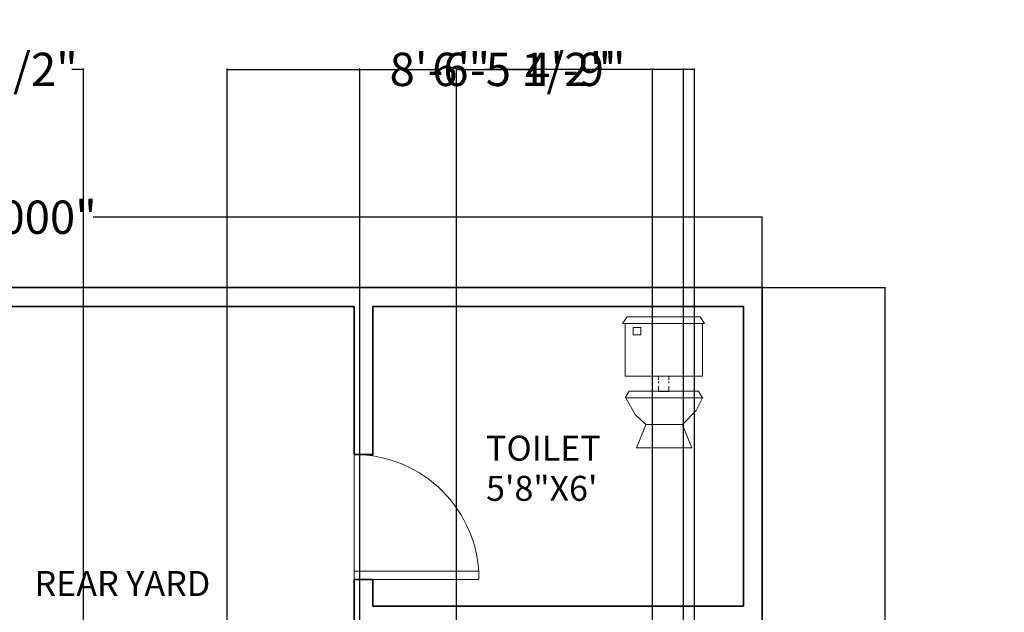
# Model space of a CAD drawing. Units: inches. Extents: x -438 to 102, y -60 to 1091.
# Tile 20 of 20: x -149 to 87, y 949 to 1091. Entities that reach past the tile are written whole.
import ezdxf

# ---------------------------------------------------------------- set-up
doc = ezdxf.new("R2010")
doc.units = ezdxf.units.IN
doc.header["$MEASUREMENT"] = 0
for name, color, linetype, lineweight, true_color in [('A-ANNO-DIMS', 217, 'Continuous', 18, 0x93278f), ('A-DOOR', 30, 'Continuous', 18, 0xf26722), ('A-WALL', 2, 'Continuous', 35, 0xf1eb1f), ('C-PROP', 2, 'Continuous', 35, 0xf1eb1f)]:
    doc.layers.add(name, color=color, linetype=linetype, lineweight=lineweight, true_color=true_color)
doc.layers.add('A-AREA-IDEN', color=4, linetype='Continuous', lineweight=18)
doc.layers.add('A-FLOR-FIXT', color=9, linetype='Continuous', lineweight=15)
doc.styles.get("Standard").update_dxf_attribs({"font": 'arial.ttf'})
doc.dimstyles.get("Standard").update_dxf_attribs({"dimtxt": 8, "dimasz": 0.18, "dimexe": 0.18, "dimexo": 0.0625, "dimgap": 0.09, "dimtad": 0, "dimtih": 1, "dimtoh": 1, "dimdec": 4, "dimzin": 0, "dimdsep": 46, "dimlunit": 3, "dimtxsty": 'Standard', "dimcen": 0.09, "dimadec": 0, "dimazin": 0, "dimtfac": 1, "dimtdec": 4, "dimtofl": 0, "dimtmove": 0, "dimatfit": 3, "dimfxl": 1, "dimtolj": 1, "dimtzin": 0, "dimarcsym": 0})

# ---------------------------------------------------------------- blocks, each defined once
blk = doc.blocks.new('*D4')
at = {"layer": 'A-ANNO-DIMS', "color": 0, "lineweight": -2, "transparency": 16777216}
for p, q in [((-354.15, 1027.06), (-354.15, 1044.09)), ((-353.97, 1043.91), (-193.57, 1043.91)), ((28.67, 1043.91), (-131.73, 1043.91)), ((28.85, 1027.06), (28.85, 1044.09))]:
    blk.add_line(p, q, dxfattribs=at)
at = {"layer": 'A-ANNO-DIMS', "color": 0, "transparency": 16777216}
for points in [[(-353.97, 1043.94), (-353.97, 1043.88), (-354.15, 1043.91)], [(28.67, 1043.94), (28.67, 1043.88), (28.85, 1043.91)]]:
    blk.add_solid(points, dxfattribs=at)
at = {"layer": 'Defpoints', "color": 0, "transparency": 16777216}
for p in [(28.85, 1043.91), (-354.15, 1027), (28.85, 1027)]:
    blk.add_point(p, dxfattribs=at)
at = {"layer": 'A-ANNO-DIMS', "color": 0, "transparency": 16777216, "insert": (-162.65, 1043.91), "char_height": 8, "attachment_point": 5}
blk.add_mtext('\\A1;31\'-11.0000"', dxfattribs=at)
blk = doc.blocks.new('*D5')
at = {"layer": 'A-ANNO-DIMS', "color": 0, "lineweight": -2, "transparency": 16777216}
for p, q in [((28.92, 1027), (58.42, 1027)), ((58.24, 1026.82), (58.24, 519.68)), ((58.24, 4.18), (58.24, 511.32)), ((28.92, 4), (58.42, 4))]:
    blk.add_line(p, q, dxfattribs=at)
at = {"layer": 'A-ANNO-DIMS', "color": 0, "transparency": 16777216}
for points in [[(58.21, 1026.82), (58.27, 1026.82), (58.24, 1027)], [(58.21, 4.18), (58.27, 4.18), (58.24, 4)]]:
    blk.add_solid(points, dxfattribs=at)
at = {"layer": 'Defpoints', "color": 0, "transparency": 16777216}
for p in [(28.85, 1027), (28.85, 4), (58.24, 4)]:
    blk.add_point(p, dxfattribs=at)
at = {"layer": 'A-ANNO-DIMS', "color": 0, "transparency": 16777216, "insert": (58.24, 515.5), "char_height": 8, "attachment_point": 5}
blk.add_mtext('\\A1;85\'-3.0000"', dxfattribs=at)
blk = doc.blocks.new('WC-CLOSE-COUPLED')
for p, q in [((-9.84, -1.66, -13.5), (-8.74, 0, -13.5)), ((-8.74, 0, -13.5), (8.78, 0, -13.5)), ((9.84, -1.66, -13.5), (8.78, 0, -13.5)), ((-9.84, -1.66, -13.5), (9.84, -1.66, -13.5)), ((-9.27, -1.66, -13.5), (-9.27, -14.26, -13.5)), ((9.31, -14.26, -13.5), (9.31, -1.66, -13.5)), ((-7.35, -2.62, -13.5), (-7.35, -4.39, -13.5)), ((-5.45, -2.62, -13.5), (-7.35, -2.62, -13.5)), ((-7.35, -4.39, -13.5), (-5.45, -4.39, -13.5)), ((-5.45, -4.39, -13.5), (-5.45, -2.62, -13.5)), ((-9.27, -14.26, -13.5), (9.31, -14.26, -13.5)), ((-1.22, -15.15, -13.5), (-1.22, -14.23, -13.5)), ((-1.22, -15.97, -13.5), (-1.22, -15.56, -13.5)), ((0.02, -14.26, -13.5), (1.26, -14.26, -13.5)), ((1.26, -14.26, -13.5), (1.26, -15.15, -13.5)), ((1.26, -15.56, -13.5), (1.26, -15.97, -13.5)), ((-9.27, -19.49, -13.5), (-8.25, -17.89, -13.5)), ((-8.25, -17.89, -13.5), (8.4, -17.89, -13.5)), ((-1.22, -17.96, -13.5), (-1.22, -16.65, -13.5)), ((1.26, -17.96, -13.5), (-1.22, -17.96, -13.5)), ((1.26, -16.65, -13.5), (1.26, -17.96, -13.5)), ((9.31, -19.49, -13.5), (8.4, -17.89, -13.5)), ((-9.27, -19.49, -13.5), (9.31, -19.49, -13.5)), ((9.52, -19.49, -13.5), (-9.07, -19.49, -13.5)), ((-9.07, -19.49, -13.5), (-6.87, -23.48, -13.5)), ((7.85, -22.5, -13.5), (9.31, -19.49, -13.5)), ((-6.87, -23.48, -13.5), (-4.26, -25.89, -13.5)), ((4.51, -25.89, -13.5), (7.85, -22.5, -13.5)), ((-6.51, -31.49, -13.5), (-4.3, -25.95, -13.5)), ((-4.26, -25.89, -13.5), (4.51, -25.89, -13.5)), ((4.51, -25.89, -13.5), (-4.26, -25.89, -13.5)), ((6.76, -31.49, -13.5), (4.55, -25.95, -13.5)), ((-6.51, -31.49, -13.5), (6.76, -31.49, -13.5)), ((0.12, -31.49, -13.5), (-6.51, -31.49, -13.5))]:
    blk.add_line(p, q)
blk = doc.blocks.new('DOOR-SWING-30')
for p, q in [((0, 0), (-30, 0)), ((0, -30), (0, 0)), ((0, -2), (-30, -2))]:
    blk.add_line(p, q)
blk.add_arc((0, 0), 30, 180, 270)
blk = doc.blocks.new('*D37')
at = {"layer": 'A-ANNO-DIMS', "color": 0, "lineweight": -2, "transparency": 16777216}
for p, q in [((-179.8, 234.94), (-179.8, 1079.58)), ((-179.62, 1079.4), (-176.98, 1079.4)), ((-134.26, 1079.4), (-136.9, 1079.4)), ((-134.08, 234.94), (-134.08, 1079.58))]:
    blk.add_line(p, q, dxfattribs=at)
at = {"layer": 'A-ANNO-DIMS', "color": 0, "transparency": 16777216}
for points in [[(-179.62, 1079.43), (-179.62, 1079.37), (-179.8, 1079.4)], [(-134.26, 1079.43), (-134.26, 1079.37), (-134.08, 1079.4)]]:
    blk.add_solid(points, dxfattribs=at)
at = {"layer": 'Defpoints', "color": 0, "transparency": 16777216}
for p in [(-134.08, 1079.4), (-179.8, 234.88), (-134.08, 234.88)]:
    blk.add_point(p, dxfattribs=at)
at = {"layer": 'A-ANNO-DIMS', "color": 0, "transparency": 16777216, "insert": (-156.94, 1079.4), "char_height": 8, "attachment_point": 5}
blk.add_mtext('\\A1;3\'-9 1/2"', dxfattribs=at)
blk = doc.blocks.new('*D45')
at = {"layer": 'A-ANNO-DIMS', "color": 0, "lineweight": -2, "transparency": 16777216}
for p, q in [((-99.58, 615.92), (-99.58, 1079.58)), ((-99.4, 1079.4), (-59.27, 1079.4)), ((2.32, 1079.4), (-37.82, 1079.4)), ((2.5, 615.92), (2.5, 1079.58))]:
    blk.add_line(p, q, dxfattribs=at)
at = {"layer": 'A-ANNO-DIMS', "color": 0, "transparency": 16777216}
for points in [[(-99.4, 1079.43), (-99.4, 1079.37), (-99.58, 1079.4)], [(2.32, 1079.43), (2.32, 1079.37), (2.5, 1079.4)]]:
    blk.add_solid(points, dxfattribs=at)
at = {"layer": 'Defpoints', "color": 0, "transparency": 16777216}
for p in [(2.5, 1079.4), (-99.58, 615.86), (2.5, 615.86)]:
    blk.add_point(p, dxfattribs=at)
at = {"layer": 'A-ANNO-DIMS', "color": 0, "transparency": 16777216, "insert": (-48.54, 1079.4), "char_height": 8, "attachment_point": 5}
blk.add_mtext('\\A1;8\'-6"', dxfattribs=at)
blk = doc.blocks.new('*D47')
at = {"layer": 'A-ANNO-DIMS', "color": 0, "lineweight": -2, "transparency": 16777216}
for p, q in [((-67.74, 529.33), (-67.74, 1079.58)), ((-67.56, 1079.4), (-48.98, 1079.4)), ((9.73, 1079.4), (-8.85, 1079.4)), ((9.91, 529.33), (9.91, 1079.58))]:
    blk.add_line(p, q, dxfattribs=at)
at = {"layer": 'A-ANNO-DIMS', "color": 0, "transparency": 16777216}
for points in [[(-67.56, 1079.43), (-67.56, 1079.37), (-67.74, 1079.4)], [(9.73, 1079.43), (9.73, 1079.37), (9.91, 1079.4)]]:
    blk.add_solid(points, dxfattribs=at)
at = {"layer": 'Defpoints', "color": 0, "transparency": 16777216}
for p in [(9.91, 1079.4), (-67.74, 529.27), (9.91, 529.27)]:
    blk.add_point(p, dxfattribs=at)
at = {"layer": 'A-ANNO-DIMS', "color": 0, "transparency": 16777216, "insert": (-28.91, 1079.4), "char_height": 8, "attachment_point": 5}
blk.add_mtext('\\A1;6\'-5 1/2"', dxfattribs=at)
blk = doc.blocks.new('*D49')
at = {"layer": 'A-ANNO-DIMS', "color": 0, "lineweight": -2, "transparency": 16777216}
for p, q in [((-44.57, 339.86), (-44.57, 1079.58)), ((-44.39, 1079.4), (-26.89, 1079.4)), ((12.37, 1079.4), (-5.13, 1079.4)), ((12.55, 312.51), (12.55, 1079.58))]:
    blk.add_line(p, q, dxfattribs=at)
at = {"layer": 'A-ANNO-DIMS', "color": 0, "transparency": 16777216}
for points in [[(-44.39, 1079.43), (-44.39, 1079.37), (-44.57, 1079.4)], [(12.37, 1079.43), (12.37, 1079.37), (12.55, 1079.4)]]:
    blk.add_solid(points, dxfattribs=at)
at = {"layer": 'Defpoints', "color": 0, "transparency": 16777216}
for p in [(12.55, 1079.4), (-44.57, 339.79), (12.55, 312.44)]:
    blk.add_point(p, dxfattribs=at)
at = {"layer": 'A-ANNO-DIMS', "color": 0, "transparency": 16777216, "insert": (-16.01, 1079.4), "char_height": 8, "attachment_point": 5}
blk.add_mtext('\\A1;4\'-9"', dxfattribs=at)

msp = doc.modelspace()

# ---------------------------------------------------------------- linework, layer by layer
at = {"layer": 'A-WALL'}
for p, q in [((-69.14649, 1022.49939), (-69.14649, 986.94813)), ((24.35351, 1022.49939), (-64.64649, 1022.49939)), ((-64.64649, 1022.49939), (-64.64649, 986.94813)), ((24.35351, 950.49939), (24.35351, 1022.49939)), ((-64.64649, 986.94813), (-69.14649, 986.94813)), ((-64.64649, 956.94813), (-69.14649, 956.94813)), ((-69.14649, 956.94813), (-69.14649, 843.99939)), ((-64.64649, 956.94813), (-64.64649, 950.49939)), ((24.35351, 950.49939), (-64.64649, 950.49939))]:
    msp.add_line(p, q, dxfattribs=at)
at = {"layer": 'C-PROP'}
for p, q in [((28.85351, 1026.99939), (-354.14649, 1026.99939)), ((28.85351, 3.99939), (28.85351, 1026.99939)), ((-69.14649, 1022.49939), (-183.14649, 1022.49939))]:
    msp.add_line(p, q, dxfattribs=at)

# ---------------------------------------------------------------- block references
at = {"layer": 'A-DOOR', "rotation": 180}
msp.add_blockref('DOOR-SWING-30', (-69.14649, 956.94813), dxfattribs=at)
at = {"layer": 'A-FLOR-FIXT'}
msp.add_blockref('WC-CLOSE-COUPLED', (5.17644, 1020.03513), dxfattribs=at)

# ---------------------------------------------------------------- texts
at = {"layer": 'A-AREA-IDEN'}
for s, p in [('TOILET', (-37.45049, 985.46368)), ('5\'8"X6\'', (-37.45049, 975.82521)), ('REAR YARD', (-145.82792, 952.97677))]:
    msp.add_text(s, height=6, dxfattribs=at).set_placement(p)

# ---------------------------------------------------------------- dimensions: what is measured, and where the dimension line sits
at = {"layer": 'A-ANNO-DIMS'}
for base, p1, p2, override, picture, middle in [((-134.07948, 1079.39939), (-179.79585, 234.87846), (-134.07948, 234.87846), {"dimdec": 1, "dimlfac": 1, "dimrnd": 0, "dimzin": 1, "dimdsep": 46, "dimlunit": 4, "dimfrac": 2}, '*D37', (-156.93767, 1079.39939)), ((9.9115, 1079.39939), (-67.73982, 529.2655), (9.9115, 529.2655), {"dimdec": 1, "dimlfac": 1, "dimrnd": 0, "dimzin": 1, "dimdsep": 46, "dimlunit": 4, "dimfrac": 2}, '*D47', (-28.91416, 1079.39939)), ((2.49567, 1079.39939), (-99.58389, 615.85716), (2.49567, 615.85716), {"dimdec": 1, "dimlfac": 1, "dimrnd": 0, "dimzin": 1, "dimdsep": 46, "dimlunit": 4, "dimfrac": 2}, '*D45', (-48.54411, 1079.39939)), ((12.55306, 1079.39939), (-44.57214, 339.79496), (12.55306, 312.44261), {"dimdec": 1, "dimlfac": 1, "dimrnd": 0, "dimzin": 1, "dimdsep": 46, "dimlunit": 4, "dimfrac": 2}, '*D49', (-16.00954, 1079.39939)), ((28.85351, 1043.90502), (-354.14649, 1026.99939), (28.85351, 1026.99939), {"dimclrd": 0, "dimclre": 0, "dimclrt": 0}, '*D4', (-162.64649, 1043.90502))]:
    dim = msp.add_linear_dim(base=base, p1=p1, p2=p2, dimstyle='Standard', override=override, dxfattribs=at)
    dim.commit()
    dim.dimension.update_dxf_attribs({"geometry": picture, "text_midpoint": middle})
dim = msp.add_linear_dim(base=(58.24207, 3.99939), p1=(28.85351, 1026.99939), p2=(28.85351, 3.99939), angle=90, dimstyle='Standard', override={"dimclrd": 0, "dimclre": 0, "dimclrt": 0}, dxfattribs=at)
dim.commit()
dim.dimension.update_dxf_attribs({"geometry": '*D5', "text_midpoint": (58.24207, 515.49939)})

doc.saveas('drawing.dxf')
